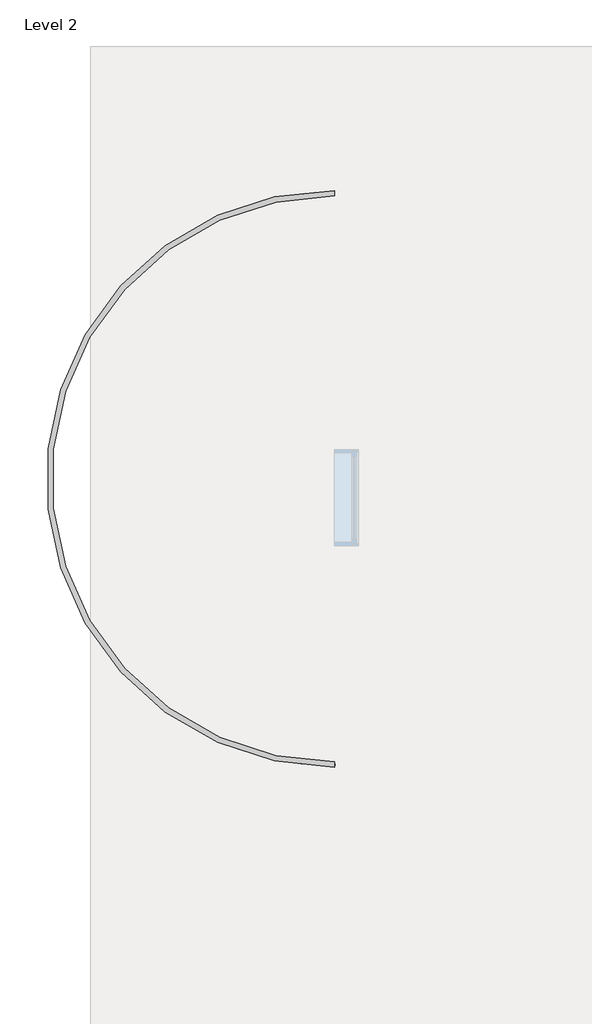
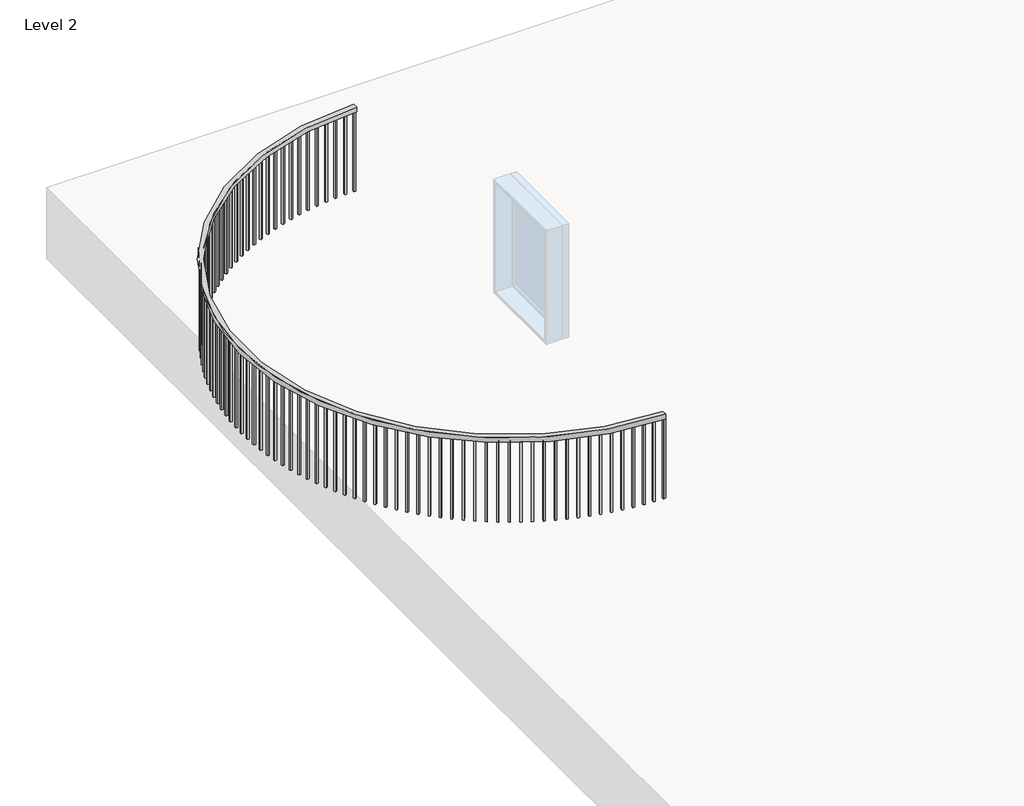
# One storey, part 2 of 2: 1 railing.
"""IFC4 building model written with IfcOpenShell, lengths in millimetres."""

from ifc_helpers import new_model, si_unit, point, frame, frame_2d, origin, place, context, project, spatial, polyline, circle_curve, trimmed, segment, composite_curve, outline, extrude, element, save

model = new_model("IFC4")

# Units and contexts
model_context = context("Model", 3, world=origin())
ifc_project = project(units=[si_unit("LENGTHUNIT", "METRE", prefix="MILLI")], contexts=[model_context])

# Site, building, storey
site = spatial("IfcSite", under=ifc_project)
building = spatial("IfcBuilding", under=site)
storey = spatial("IfcBuildingStorey", under=building, Name="Level 2", Elevation=3048.0)

# Railing
placement = place(None, origin())
element("IfcRailing", 1, ObjectType="Handrail - Rectangular", at=placement, inside=storey, context=model_context, shape_type="SweptSolid", body=[
    extrude(outline(composite_curve([segment(trimmed(circle_curve(frame_2d((-15728.6368919, 10326.9945075)), 2743.2), [point((-15728.6368919, 7583.7945075))], [point((-15728.6368919, 13070.1945075))], False, "CARTESIAN"), True, "CONTINUOUS"), segment(polyline([(-15728.6368919, 13070.1945075), (-15728.6368919, 13019.3945075)]), True, "CONTINUOUS"), segment(trimmed(circle_curve(frame_2d((-15728.6368919, 10326.9945075)), 2692.4), [point((-15728.6368919, 13019.3945075))], [point((-15728.6368919, 7634.5945075))], True, "CARTESIAN"), True, "CONTINUOUS"), segment(polyline([(-15728.6368919, 7634.5945075), (-15728.6368919, 7583.7945075)]), True, "CONTINUOUS")], self_intersect=False)), frame((0.0, 0.0, 3911.6), z_axis=(0.0, 0.0, 1.0), x_axis=(1.0, 0.0, 0.0)), (0.0, 0.0, 1.0), 50.8),
    extrude(outline(polyline([(-15741.9957848, 7599.6855919), (-15741.9690055, 7618.735573), (-15722.9190243, 7618.7087937), (-15722.9458036, 7599.6588126), (-15741.9957848, 7599.6855919)])), frame((0.0, 0.0, 3048.0), z_axis=(0.0, 0.0, 1.0), x_axis=(1.0, 0.0, 0.0)), (0.0, 0.0, 1.0), 863.6),
    extrude(outline(polyline([(-15843.9181793, 7602.0903613), (-15843.1794358, 7621.1260319), (-15824.1437651, 7620.3872884), (-15824.8825087, 7601.3516177), (-15843.9181793, 7602.0903613)])), frame((0.0, 0.0, 3048.0), z_axis=(0.0, 0.0, 1.0), x_axis=(1.0, 0.0, 0.0)), (0.0, 0.0, 1.0), 863.6),
    extrude(outline(polyline([(-15945.6794868, 7608.3027461), (-15944.2298113, 7627.297507), (-15925.2350504, 7625.8478315), (-15926.6847259, 7606.8530706), (-15945.6794868, 7608.3027461)])), frame((0.0, 0.0, 3048.0), z_axis=(0.0, 0.0, 1.0), x_axis=(1.0, 0.0, 0.0)), (0.0, 0.0, 1.0), 863.6),
    extrude(outline(polyline([(-16047.1375121, 7618.3140656), (-16044.9789303, 7637.2413746), (-16026.0516213, 7635.0827927), (-16028.2102032, 7616.1554838), (-16047.1375121, 7618.3140656)])), frame((0.0, 0.0, 3048.0), z_axis=(0.0, 0.0, 1.0), x_axis=(1.0, 0.0, 0.0)), (0.0, 0.0, 1.0), 863.6),
    extrude(outline(polyline([(-16148.150484, 7632.1103305), (-16145.2860122, 7650.9437397), (-16126.452603, 7648.0792678), (-16129.3170749, 7629.2458587), (-16148.150484, 7632.1103305)])), frame((0.0, 0.0, 3048.0), z_axis=(0.0, 0.0, 1.0), x_axis=(1.0, 0.0, 0.0)), (0.0, 0.0, 1.0), 863.6),
    extrude(outline(polyline([(-16248.5772532, 7649.6722628), (-16245.0108939, 7668.3854555), (-16226.2977012, 7664.8190963), (-16229.8640605, 7646.1059035), (-16248.5772532, 7649.6722628)])), frame((0.0, 0.0, 3048.0), z_axis=(0.0, 0.0, 1.0), x_axis=(1.0, 0.0, 0.0)), (0.0, 0.0, 1.0), 863.6),
    extrude(outline(polyline([(-16348.2774892, 7670.9753224), (-16344.014226, 7689.54215), (-16325.4473984, 7685.2788868), (-16329.7106616, 7666.7120592), (-16348.2774892, 7670.9753224)])), frame((0.0, 0.0, 3048.0), z_axis=(0.0, 0.0, 1.0), x_axis=(1.0, 0.0, 0.0)), (0.0, 0.0, 1.0), 863.6),
    extrude(outline(polyline([(-16447.1118772, 7695.9897418), (-16442.1576672, 7714.3842602), (-16423.7631489, 7709.4300502), (-16428.7173589, 7691.0355319), (-16447.1118772, 7695.9897418)])), frame((0.0, 0.0, 3048.0), z_axis=(0.0, 0.0, 1.0), x_axis=(1.0, 0.0, 0.0)), (0.0, 0.0, 1.0), 863.6),
    extrude(outline(polyline([(-16544.9423119, 7724.6805674), (-16539.3040779, 7742.8770731), (-16521.1075722, 7737.2388391), (-16526.7458062, 7719.0423334), (-16544.9423119, 7724.6805674)])), frame((0.0, 0.0, 3048.0), z_axis=(0.0, 0.0, 1.0), x_axis=(1.0, 0.0, 0.0)), (0.0, 0.0, 1.0), 863.6),
    extrude(outline(polyline([(-16641.632091, 7757.0077083), (-16635.3177115, 7774.9807746), (-16617.3446452, 7768.6663951), (-16623.6590247, 7750.6933288), (-16641.632091, 7757.0077083)])), frame((0.0, 0.0, 3048.0), z_axis=(0.0, 0.0, 1.0), x_axis=(1.0, 0.0, 0.0)), (0.0, 0.0, 1.0), 863.6),
    extrude(outline(polyline([(-16737.0461061, 7792.9259926), (-16730.0644044, 7810.6505051), (-16712.3398919, 7803.6688034), (-16719.3215936, 7785.9442909), (-16737.0461061, 7792.9259926)])), frame((0.0, 0.0, 3048.0), z_axis=(0.0, 0.0, 1.0), x_axis=(1.0, 0.0, 0.0)), (0.0, 0.0, 1.0), 863.6),
    extrude(outline(polyline([(-16831.0510314, 7832.3852302), (-16823.4117634, 7849.8364217), (-16805.9605719, 7842.1971536), (-16813.59984, 7824.7459621), (-16831.0510314, 7832.3852302)])), frame((0.0, 0.0, 3048.0), z_axis=(0.0, 0.0, 1.0), x_axis=(1.0, 0.0, 0.0)), (0.0, 0.0, 1.0), 863.6),
    extrude(outline(polyline([(-16923.5155103, 7875.3302832), (-16915.2293505, 7892.4837684), (-16898.0758652, 7884.1976086), (-16906.362025, 7867.0441234), (-16923.5155103, 7875.3302832)])), frame((0.0, 0.0, 3048.0), z_axis=(0.0, 0.0, 1.0), x_axis=(1.0, 0.0, 0.0)), (0.0, 0.0, 1.0), 863.6),
    extrude(outline(polyline([(-17014.3103383, 7921.7011427), (-17005.3888654, 7938.5329525), (-16988.5570556, 7929.6114796), (-16997.4785285, 7912.7796698), (-17014.3103383, 7921.7011427)])), frame((0.0, 0.0, 3048.0), z_axis=(0.0, 0.0, 1.0), x_axis=(1.0, 0.0, 0.0)), (0.0, 0.0, 1.0), 863.6),
    extrude(outline(polyline([(-17103.3086445, 7971.4330131), (-17093.7643247, 7987.9196276), (-17077.2777101, 7978.3753079), (-17086.8220299, 7961.8886933), (-17103.3086445, 7971.4330131)])), frame((0.0, 0.0, 3048.0), z_axis=(0.0, 0.0, 1.0), x_axis=(1.0, 0.0, 0.0)), (0.0, 0.0, 1.0), 863.6),
    extrude(outline(polyline([(-17190.3860679, 8024.4564019), (-17180.2322379, 8040.5747838), (-17164.1138559, 8030.4209539), (-17174.2676859, 8014.3025719), (-17190.3860679, 8024.4564019)])), frame((0.0, 0.0, 3048.0), z_axis=(0.0, 0.0, 1.0), x_axis=(1.0, 0.0, 0.0)), (0.0, 0.0, 1.0), 863.6),
    extrude(outline(polyline([(-17275.4209318, 8080.6972174), (-17264.67178, 8096.424844), (-17248.9441535, 8085.6756922), (-17259.6933053, 8069.9480657), (-17275.4209318, 8080.6972174)])), frame((0.0, 0.0, 3048.0), z_axis=(0.0, 0.0, 1.0), x_axis=(1.0, 0.0, 0.0)), (0.0, 0.0, 1.0), 863.6),
    extrude(outline(polyline([(-17358.2944137, 8140.0768723), (-17346.9649603, 8155.3917666), (-17331.6500661, 8144.0623132), (-17342.9795194, 8128.747419), (-17358.2944137, 8140.0768723)])), frame((0.0, 0.0, 3048.0), z_axis=(0.0, 0.0, 1.0), x_axis=(1.0, 0.0, 0.0)), (0.0, 0.0, 1.0), 863.6),
    extrude(outline(polyline([(-17438.8907113, 8202.512393), (-17426.9967874, 8217.3931549), (-17412.1160255, 8205.499231), (-17424.0099494, 8190.6184691), (-17438.8907113, 8202.512393)])), frame((0.0, 0.0, 3048.0), z_axis=(0.0, 0.0, 1.0), x_axis=(1.0, 0.0, 0.0)), (0.0, 0.0, 1.0), 863.6),
    extrude(outline(polyline([(-17517.0972041, 8267.9165359), (-17504.6554295, 8282.3423719), (-17490.2295935, 8269.9005973), (-17502.671368, 8255.4747613), (-17517.0972041, 8267.9165359)])), frame((0.0, 0.0, 3048.0), z_axis=(0.0, 0.0, 1.0), x_axis=(1.0, 0.0, 0.0)), (0.0, 0.0, 1.0), 863.6),
    extrude(outline(polyline([(-17592.8046111, 8336.1979092), (-17579.8323713, 8350.1486616), (-17565.8816189, 8337.1764217), (-17578.8538587, 8323.2256693), (-17592.8046111, 8336.1979092)])), frame((0.0, 0.0, 3048.0), z_axis=(0.0, 0.0, 1.0), x_axis=(1.0, 0.0, 0.0)), (0.0, 0.0, 1.0), 863.6),
    extrude(outline(polyline([(-17665.9071435, 8407.2611006), (-17652.422565, 8420.7172754), (-17638.9663901, 8407.2326969), (-17652.4509687, 8393.7765221), (-17665.9071435, 8407.2611006)])), frame((0.0, 0.0, 3048.0), z_axis=(0.0, 0.0, 1.0), x_axis=(1.0, 0.0, 0.0)), (0.0, 0.0, 1.0), 863.6),
    extrude(outline(polyline([(-17736.3026522, 8481.0068109), (-17722.3245775, 8493.9496053), (-17709.3817831, 8479.9715306), (-17723.3598578, 8467.0287361), (-17736.3026522, 8481.0068109)])), frame((0.0, 0.0, 3048.0), z_axis=(0.0, 0.0, 1.0), x_axis=(1.0, 0.0, 0.0)), (0.0, 0.0, 1.0), 863.6),
    extrude(outline(polyline([(-17803.8927708, 8557.3319921), (-17789.4407321, 8569.7433206), (-17777.0294035, 8555.2912819), (-17791.4814423, 8542.8799533), (-17803.8927708, 8557.3319921)])), frame((0.0, 0.0, 3048.0), z_axis=(0.0, 0.0, 1.0), x_axis=(1.0, 0.0, 0.0)), (0.0, 0.0, 1.0), 863.6),
    extrude(outline(polyline([(-17868.583053, 8636.1299922), (-17853.6772446, 8647.992512), (-17841.8147248, 8633.0867036), (-17856.7205331, 8621.2241838), (-17868.583053, 8636.1299922)])), frame((0.0, 0.0, 3048.0), z_axis=(0.0, 0.0, 1.0), x_axis=(1.0, 0.0, 0.0)), (0.0, 0.0, 1.0), 863.6),
    extrude(outline(polyline([(-17930.2831044, 8717.2907036), (-17914.9443548, 8728.5878387), (-17903.6472197, 8713.2490891), (-17918.9859693, 8701.951954), (-17930.2831044, 8717.2907036)])), frame((0.0, 0.0, 3048.0), z_axis=(0.0, 0.0, 1.0), x_axis=(1.0, 0.0, 0.0)), (0.0, 0.0, 1.0), 863.6),
    extrude(outline(polyline([(-17988.9067092, 8800.7007172), (-17973.1564519, 8811.4166817), (-17962.4404874, 8795.6664245), (-17978.1907447, 8784.9504599), (-17988.9067092, 8800.7007172)])), frame((0.0, 0.0, 3048.0), z_axis=(0.0, 0.0, 1.0), x_axis=(1.0, 0.0, 0.0)), (0.0, 0.0, 1.0), 863.6),
    extrude(outline(polyline([(-18044.3719504, 8886.2434811), (-18028.2321938, 8896.3633011), (-18018.1123738, 8880.2235446), (-18034.2521303, 8870.1037245), (-18044.3719504, 8886.2434811)])), frame((0.0, 0.0, 3048.0), z_axis=(0.0, 0.0, 1.0), x_axis=(1.0, 0.0, 0.0)), (0.0, 0.0, 1.0), 863.6),
    extrude(outline(polyline([(-18096.6013241, 8973.7994628), (-18080.094621, 8983.3089976), (-18070.5850862, 8966.8022945), (-18087.0917894, 8957.2927597), (-18096.6013241, 8973.7994628)])), frame((0.0, 0.0, 3048.0), z_axis=(0.0, 0.0, 1.0), x_axis=(1.0, 0.0, 0.0)), (0.0, 0.0, 1.0), 863.6),
    extrude(outline(polyline([(-18145.5218483, 9063.2463171), (-18128.6712641, 9072.1322785), (-18119.7853026, 9055.2816943), (-18136.6358868, 9046.3957328), (-18145.5218483, 9063.2463171)])), frame((0.0, 0.0, 3048.0), z_axis=(0.0, 0.0, 1.0), x_axis=(1.0, 0.0, 0.0)), (0.0, 0.0, 1.0), 863.6),
    extrude(outline(polyline([(-18191.0651643, 9154.4590562), (-18173.894245, 9162.7090277), (-18165.6442735, 9145.5381083), (-18182.8151929, 9137.2881369), (-18191.0651643, 9154.4590562)])), frame((0.0, 0.0, 3048.0), z_axis=(0.0, 0.0, 1.0), x_axis=(1.0, 0.0, 0.0)), (0.0, 0.0, 1.0), 863.6),
    extrude(outline(polyline([(-18233.1676328, 9247.3102252), (-18215.7003719, 9254.9126786), (-18208.0979185, 9237.4454177), (-18225.5651793, 9229.8429643), (-18233.1676328, 9247.3102252)])), frame((0.0, 0.0, 3048.0), z_axis=(0.0, 0.0, 1.0), x_axis=(1.0, 0.0, 0.0)), (0.0, 0.0, 1.0), 863.6),
    extrude(outline(polyline([(-18271.7704221, 9341.6700793), (-18254.0312274, 9348.6143915), (-18247.0869153, 9330.8751968), (-18264.82611, 9323.9308846), (-18271.7704221, 9341.6700793)])), frame((0.0, 0.0, 3048.0), z_axis=(0.0, 0.0, 1.0), x_axis=(1.0, 0.0, 0.0)), (0.0, 0.0, 1.0), 863.6),
    extrude(outline(polyline([(-18306.8195913, 9437.4067659), (-18288.8332504, 9443.6832333), (-18282.5567831, 9425.6968925), (-18300.5431239, 9419.4204251), (-18306.8195913, 9437.4067659)])), frame((0.0, 0.0, 3048.0), z_axis=(0.0, 0.0, 1.0), x_axis=(1.0, 0.0, 0.0)), (0.0, 0.0, 1.0), 863.6),
    extrude(outline(polyline([(-18338.2661646, 9534.3865084), (-18320.0578106, 9539.9863606), (-18314.4579584, 9521.7780066), (-18332.6663124, 9516.1781544), (-18338.2661646, 9534.3865084)])), frame((0.0, 0.0, 3048.0), z_axis=(0.0, 0.0, 1.0), x_axis=(1.0, 0.0, 0.0)), (0.0, 0.0, 1.0), 863.6),
    extrude(outline(polyline([(-18366.0662006, 9632.4737931), (-18347.6612768, 9637.3892053), (-18342.7458646, 9618.9842814), (-18361.1507885, 9614.0688692), (-18366.0662006, 9632.4737931)])), frame((0.0, 0.0, 3048.0), z_axis=(0.0, 0.0, 1.0), x_axis=(1.0, 0.0, 0.0)), (0.0, 0.0, 1.0), 863.6),
    extrude(outline(polyline([(-18390.1808532, 9731.5315588), (-18371.6050774, 9735.7556625), (-18367.3809737, 9717.1798866), (-18385.9567496, 9712.955783), (-18390.1808532, 9731.5315588)])), frame((0.0, 0.0, 3048.0), z_axis=(0.0, 0.0, 1.0), x_axis=(1.0, 0.0, 0.0)), (0.0, 0.0, 1.0), 863.6),
    extrude(outline(polyline([(-18410.576426, 9831.4213883), (-18391.8557549, 9834.9482809), (-18388.3288623, 9816.2276097), (-18407.0495335, 9812.7007171), (-18410.576426, 9831.4213883)])), frame((0.0, 0.0, 3048.0), z_axis=(0.0, 0.0, 1.0), x_axis=(1.0, 0.0, 0.0)), (0.0, 0.0, 1.0), 863.6),
    extrude(outline(polyline([(-18427.2244196, 9932.0037015), (-18408.3850122, 9934.8284548), (-18405.560259, 9915.9890475), (-18424.3996663, 9913.1642942), (-18427.2244196, 9932.0037015)])), frame((0.0, 0.0, 3048.0), z_axis=(0.0, 0.0, 1.0), x_axis=(1.0, 0.0, 0.0)), (0.0, 0.0, 1.0), 863.6),
    extrude(outline(polyline([(-18440.1015709, 10033.1379509), (-18421.1697524, 10035.2566177), (-18419.0510856, 10016.3247992), (-18437.9829041, 10014.2061324), (-18440.1015709, 10033.1379509)])), frame((0.0, 0.0, 3048.0), z_axis=(0.0, 0.0, 1.0), x_axis=(1.0, 0.0, 0.0)), (0.0, 0.0, 1.0), 863.6),
    extrude(outline(polyline([(-18449.1898863, 10134.6828176), (-18430.1921108, 10136.0924374), (-18428.782491, 10117.094662), (-18447.7802664, 10115.6850421), (-18449.1898863, 10134.6828176)])), frame((0.0, 0.0, 3048.0), z_axis=(0.0, 0.0, 1.0), x_axis=(1.0, 0.0, 0.0)), (0.0, 0.0, 1.0), 863.6),
    extrude(outline(polyline([(-18454.4766663, 10236.4964089), (-18435.4394802, 10237.1950121), (-18434.740877, 10218.157826), (-18453.7780631, 10217.4592228), (-18454.4766663, 10236.4964089)])), frame((0.0, 0.0, 3048.0), z_axis=(0.0, 0.0, 1.0), x_axis=(1.0, 0.0, 0.0)), (0.0, 0.0, 1.0), 863.6),
    extrude(outline(polyline([(-18455.9545234, 10338.4364568), (-18436.9045281, 10338.4230671), (-18436.9179178, 10319.3730718), (-18455.967913, 10319.3864615), (-18455.9545234, 10338.4364568)])), frame((0.0, 0.0, 3048.0), z_axis=(0.0, 0.0, 1.0), x_axis=(1.0, 0.0, 0.0)), (0.0, 0.0, 1.0), 863.6),
    extrude(outline(polyline([(-18453.6213926, 10440.3605163), (-18434.5852074, 10439.6351526), (-18435.3105712, 10420.5989673), (-18454.3467564, 10421.3243311), (-18453.6213926, 10440.3605163)])), frame((0.0, 0.0, 3048.0), z_axis=(0.0, 0.0, 1.0), x_axis=(1.0, 0.0, 0.0)), (0.0, 0.0, 1.0), 863.6),
    extrude(outline(polyline([(-18447.4805342, 10542.1261652), (-18428.4847591, 10540.6898408), (-18429.9210834, 10521.6940657), (-18448.9168585, 10523.13039), (-18447.4805342, 10542.1261652)])), frame((0.0, 0.0, 3048.0), z_axis=(0.0, 0.0, 1.0), x_axis=(1.0, 0.0, 0.0)), (0.0, 0.0, 1.0), 863.6),
    extrude(outline(polyline([(-18437.5405288, 10643.5912021), (-18418.6117074, 10641.4459242), (-18420.7569852, 10622.5171027), (-18439.6858067, 10624.6623806), (-18437.5405288, 10643.5912021)])), frame((0.0, 0.0, 3048.0), z_axis=(0.0, 0.0, 1.0), x_axis=(1.0, 0.0, 0.0)), (0.0, 0.0, 1.0), 863.6),
    extrude(outline(polyline([(-18423.8152662, 10744.613846), (-18404.9798483, 10741.7626123), (-18407.8310821, 10722.9271944), (-18426.6664999, 10725.7784281), (-18423.8152662, 10744.613846)])), frame((0.0, 0.0, 3048.0), z_axis=(0.0, 0.0, 1.0), x_axis=(1.0, 0.0, 0.0)), (0.0, 0.0, 1.0), 863.6),
    extrude(outline(polyline([(-18406.3239251, 10845.0529341), (-18387.6082304, 10841.4997286), (-18391.1614358, 10822.7840338), (-18409.8771306, 10826.3372393), (-18406.3239251, 10845.0529341)])), frame((0.0, 0.0, 3048.0), z_axis=(0.0, 0.0, 1.0), x_axis=(1.0, 0.0, 0.0)), (0.0, 0.0, 1.0), 863.6),
    extrude(outline(polyline([(-18385.0909469, 10944.7681188), (-18366.5211274, 10940.5179066), (-18370.7713395, 10921.9480871), (-18389.341159, 10926.1982992), (-18385.0909469, 10944.7681188)])), frame((0.0, 0.0, 3048.0), z_axis=(0.0, 0.0, 1.0), x_axis=(1.0, 0.0, 0.0)), (0.0, 0.0, 1.0), 863.6),
    extrude(outline(polyline([(-18360.1460013, 11043.6200641), (-18341.7480054, 11038.6787843), (-18346.6892852, 11020.2807884), (-18365.0872811, 11025.2220682), (-18360.1460013, 11043.6200641)])), frame((0.0, 0.0, 3048.0), z_axis=(0.0, 0.0, 1.0), x_axis=(1.0, 0.0, 0.0)), (0.0, 0.0, 1.0), 863.6),
    extrude(outline(polyline([(-18331.5239448, 11141.4706405), (-18313.3234807, 11135.8451977), (-18318.9489235, 11117.6447336), (-18337.1493876, 11123.2701765), (-18331.5239448, 11141.4706405)])), frame((0.0, 0.0, 3048.0), z_axis=(0.0, 0.0, 1.0), x_axis=(1.0, 0.0, 0.0)), (0.0, 0.0, 1.0), 863.6),
    extrude(outline(polyline([(-18299.2647721, 11238.1831175), (-18281.287272, 11231.8813723), (-18287.5890173, 11213.9038722), (-18305.5665173, 11220.2056175), (-18299.2647721, 11238.1831175)])), frame((0.0, 0.0, 3048.0), z_axis=(0.0, 0.0, 1.0), x_axis=(1.0, 0.0, 0.0)), (0.0, 0.0, 1.0), 863.6),
    extrude(outline(polyline([(-18263.4135602, 11333.6223549), (-18245.6841449, 11326.6531129), (-18252.6533869, 11308.9236976), (-18270.3828021, 11315.8929396), (-18263.4135602, 11333.6223549)])), frame((0.0, 0.0, 3048.0), z_axis=(0.0, 0.0, 1.0), x_axis=(1.0, 0.0, 0.0)), (0.0, 0.0, 1.0), 863.6),
    extrude(outline(polyline([(-18224.0204055, 11427.6549917), (-18206.5638489, 11420.0279914), (-18214.1908492, 11402.5714348), (-18231.6474057, 11410.1984351), (-18224.0204055, 11427.6549917)])), frame((0.0, 0.0, 3048.0), z_axis=(0.0, 0.0, 1.0), x_axis=(1.0, 0.0, 0.0)), (0.0, 0.0, 1.0), 863.6),
    extrude(outline(polyline([(-18181.1403535, 11520.1496324), (-18163.9810484, 11511.8755313), (-18172.2551495, 11494.7162262), (-18189.4144546, 11502.9903273), (-18181.1403535, 11520.1496324)])), frame((0.0, 0.0, 3048.0), z_axis=(0.0, 0.0, 1.0), x_axis=(1.0, 0.0, 0.0)), (0.0, 0.0, 1.0), 863.6),
    extrude(outline(polyline([(-18134.8333222, 11610.9770307), (-18117.995246, 11602.0673905), (-18126.9048862, 11585.2293142), (-18143.7429624, 11594.1389544), (-18134.8333222, 11610.9770307)])), frame((0.0, 0.0, 3048.0), z_axis=(0.0, 0.0, 1.0), x_axis=(1.0, 0.0, 0.0)), (0.0, 0.0, 1.0), 863.6),
    extrude(outline(polyline([(-18085.1640183, 11700.0102698), (-18068.6706994, 11690.4775403), (-18078.2034289, 11673.9842214), (-18094.6967478, 11683.5169509), (-18085.1640183, 11700.0102698)])), frame((0.0, 0.0, 3048.0), z_axis=(0.0, 0.0, 1.0), x_axis=(1.0, 0.0, 0.0)), (0.0, 0.0, 1.0), 863.6),
    extrude(outline(polyline([(-18032.2018467, 11787.1249402), (-18016.0763318, 11776.9824419), (-18026.2188302, 11760.8569271), (-18042.344345, 11770.9994254), (-18032.2018467, 11787.1249402)])), frame((0.0, 0.0, 3048.0), z_axis=(0.0, 0.0, 1.0), x_axis=(1.0, 0.0, 0.0)), (0.0, 0.0, 1.0), 863.6),
    extrude(outline(polyline([(-17976.0208133, 11872.199313), (-17960.2856354, 11861.4612184), (-17971.0237301, 11845.7260405), (-17986.758908, 11856.4641351), (-17976.0208133, 11872.199313)])), frame((0.0, 0.0, 3048.0), z_axis=(0.0, 0.0, 1.0), x_axis=(1.0, 0.0, 0.0)), (0.0, 0.0, 1.0), 863.6),
    extrude(outline(polyline([(-17916.6994223, 11955.1145106), (-17901.3765687, 11943.7958244), (-17912.6952549, 11928.4729708), (-17928.0181085, 11939.791657), (-17916.6994223, 11955.1145106)])), frame((0.0, 0.0, 3048.0), z_axis=(0.0, 0.0, 1.0), x_axis=(1.0, 0.0, 0.0)), (0.0, 0.0, 1.0), 863.6),
    extrude(outline(polyline([(-17854.3205656, 12035.7546722), (-17839.4314475, 12023.8712105), (-17851.3149093, 12008.9820924), (-17866.2040274, 12020.8655541), (-17854.3205656, 12035.7546722)])), frame((0.0, 0.0, 3048.0), z_axis=(0.0, 0.0, 1.0), x_axis=(1.0, 0.0, 0.0)), (0.0, 0.0, 1.0), 863.6),
    extrude(outline(polyline([(-17788.9714078, 12114.0071162), (-17774.5368304, 12101.5754842), (-17786.9684624, 12087.1409068), (-17801.4030399, 12099.5725388), (-17788.9714078, 12114.0071162)])), frame((0.0, 0.0, 3048.0), z_axis=(0.0, 0.0, 1.0), x_axis=(1.0, 0.0, 0.0)), (0.0, 0.0, 1.0), 863.6),
    extrude(outline(polyline([(-17720.7432638, 12189.7624974), (-17706.783397, 12176.8000663), (-17719.7458282, 12162.8401996), (-17733.7056949, 12175.8026307), (-17720.7432638, 12189.7624974)])), frame((0.0, 0.0, 3048.0), z_axis=(0.0, 0.0, 1.0), x_axis=(1.0, 0.0, 0.0)), (0.0, 0.0, 1.0), 863.6),
    extrude(outline(polyline([(-17649.7314714, 12262.9149599), (-17636.265822, 12249.4398426), (-17649.7409393, 12235.9741932), (-17663.2065887, 12249.4493105), (-17649.7314714, 12262.9149599)])), frame((0.0, 0.0, 3048.0), z_axis=(0.0, 0.0, 1.0), x_axis=(1.0, 0.0, 0.0)), (0.0, 0.0, 1.0), 863.6),
    extrude(outline(polyline([(-17576.0352582, 12333.3622847), (-17563.0826422, 12319.3933106), (-17577.0516164, 12306.4406946), (-17590.0042323, 12320.4096688), (-17576.0352582, 12333.3622847)])), frame((0.0, 0.0, 3048.0), z_axis=(0.0, 0.0, 1.0), x_axis=(1.0, 0.0, 0.0)), (0.0, 0.0, 1.0), 863.6),
    extrude(outline(polyline([(-17499.7576028, 12401.0060332), (-17487.3361194, 12386.5627216), (-17501.779431, 12374.1412382), (-17514.2009144, 12388.5845499), (-17499.7576028, 12401.0060332)])), frame((0.0, 0.0, 3048.0), z_axis=(0.0, 0.0, 1.0), x_axis=(1.0, 0.0, 0.0)), (0.0, 0.0, 1.0), 863.6),
    extrude(outline(polyline([(-17421.0050909, 12465.751684), (-17409.1320972, 12450.8542171), (-17424.0295641, 12438.9812234), (-17435.9025578, 12453.8786903), (-17421.0050909, 12465.751684)])), frame((0.0, 0.0, 3048.0), z_axis=(0.0, 0.0, 1.0), x_axis=(1.0, 0.0, 0.0)), (0.0, 0.0, 1.0), 863.6),
    extrude(outline(polyline([(-17339.8877666, 12527.5087656), (-17328.5798531, 12512.1779602), (-17343.9106585, 12500.8700467), (-17355.218572, 12516.2008521), (-17339.8877666, 12527.5087656)])), frame((0.0, 0.0, 3048.0), z_axis=(0.0, 0.0, 1.0), x_axis=(1.0, 0.0, 0.0)), (0.0, 0.0, 1.0), 863.6),
    extrude(outline(polyline([(-17256.5189783, 12586.1909822), (-17245.791946, 12570.4482607), (-17261.5346675, 12559.7212285), (-17272.2616997, 12575.46395), (-17256.5189783, 12586.1909822)])), frame((0.0, 0.0, 3048.0), z_axis=(0.0, 0.0, 1.0), x_axis=(1.0, 0.0, 0.0)), (0.0, 0.0, 1.0), 863.6),
    extrude(outline(polyline([(-17171.0152203, 12641.716335), (-17160.8840587, 12625.5836953), (-17177.0166983, 12615.4525337), (-17187.14786, 12631.5851733), (-17171.0152203, 12641.716335)])), frame((0.0, 0.0, 3048.0), z_axis=(0.0, 0.0, 1.0), x_axis=(1.0, 0.0, 0.0)), (0.0, 0.0, 1.0), 863.6),
    extrude(outline(polyline([(-17083.4959706, 12694.0072362), (-17073.9748361, 12677.5072211), (-17090.4748512, 12667.9860867), (-17099.9959857, 12684.4861018), (-17083.4959706, 12694.0072362)])), frame((0.0, 0.0, 3048.0), z_axis=(0.0, 0.0, 1.0), x_axis=(1.0, 0.0, 0.0)), (0.0, 0.0, 1.0), 863.6),
    extrude(outline(polyline([(-16994.0835232, 12742.9906177), (-16985.1857201, 12726.1462833), (-17002.0300546, 12717.2484803), (-17010.9278576, 12734.0928147), (-16994.0835232, 12742.9906177)])), frame((0.0, 0.0, 3048.0), z_axis=(0.0, 0.0, 1.0), x_axis=(1.0, 0.0, 0.0)), (0.0, 0.0, 1.0), 863.6),
    extrude(outline(polyline([(-16902.9028175, 12788.5980331), (-16894.6407792, 12771.4329166), (-16911.8058957, 12763.1708783), (-16920.067934, 12780.3359948), (-16902.9028175, 12788.5980331)])), frame((0.0, 0.0, 3048.0), z_axis=(0.0, 0.0, 1.0), x_axis=(1.0, 0.0, 0.0)), (0.0, 0.0, 1.0), 863.6),
    extrude(outline(polyline([(-16810.081264, 12830.7657533), (-16802.4665353, 12813.3038403), (-16819.9284483, 12805.6891115), (-16827.543177, 12823.1510246), (-16810.081264, 12830.7657533)])), frame((0.0, 0.0, 3048.0), z_axis=(0.0, 0.0, 1.0), x_axis=(1.0, 0.0, 0.0)), (0.0, 0.0, 1.0), 863.6),
    extrude(outline(polyline([(-16715.7485659, 12869.4348557), (-16708.7917871, 12851.7005464), (-16726.5260965, 12844.7437676), (-16733.4828752, 12862.4780769), (-16715.7485659, 12869.4348557)])), frame((0.0, 0.0, 3048.0), z_axis=(0.0, 0.0, 1.0), x_axis=(1.0, 0.0, 0.0)), (0.0, 0.0, 1.0), 863.6),
    extrude(outline(polyline([(-16620.0365379, 12904.5513065), (-16613.74743, 12886.5693817), (-16631.7293549, 12880.2802738), (-16638.0184627, 12898.2621987), (-16620.0365379, 12904.5513065)])), frame((0.0, 0.0, 3048.0), z_axis=(0.0, 0.0, 1.0), x_axis=(1.0, 0.0, 0.0)), (0.0, 0.0, 1.0), 863.6),
    extrude(outline(polyline([(-16523.0789222, 12936.0660362), (-16517.4662733, 12917.8616226), (-16535.6706868, 12912.2489737), (-16541.2833357, 12930.4533872), (-16523.0789222, 12936.0660362)])), frame((0.0, 0.0, 3048.0), z_axis=(0.0, 0.0, 1.0), x_axis=(1.0, 0.0, 0.0)), (0.0, 0.0, 1.0), 863.6),
    extrude(outline(polyline([(-16425.0112015, 12963.9350078), (-16420.0828543, 12945.5335433), (-16438.4843187, 12940.6051961), (-16443.4126659, 12959.0066606), (-16425.0112015, 12963.9350078)])), frame((0.0, 0.0, 3048.0), z_axis=(0.0, 0.0, 1.0), x_axis=(1.0, 0.0, 0.0)), (0.0, 0.0, 1.0), 863.6),
    extrude(outline(polyline([(-16325.9704097, 12988.119279), (-16321.7332507, 12969.5464768), (-16340.306053, 12965.3093178), (-16344.5432119, 12983.8821201), (-16325.9704097, 12988.119279)])), frame((0.0, 0.0, 3048.0), z_axis=(0.0, 0.0, 1.0), x_axis=(1.0, 0.0, 0.0)), (0.0, 0.0, 1.0), 863.6),
    extrude(outline(polyline([(-16226.0949403, 13008.5850563), (-16222.5548904, 12989.8668687), (-16241.273078, 12986.3268188), (-16244.8131279, 13005.0450064), (-16226.0949403, 13008.5850563)])), frame((0.0, 0.0, 3048.0), z_axis=(0.0, 0.0, 1.0), x_axis=(1.0, 0.0, 0.0)), (0.0, 0.0, 1.0), 863.6),
    extrude(outline(polyline([(-16125.5243533, 13025.3037418), (-16122.686359, 13006.4663246), (-16141.5237763, 13003.6283304), (-16144.3617705, 13022.4657476), (-16125.5243533, 13025.3037418)])), frame((0.0, 0.0, 3048.0), z_axis=(0.0, 0.0, 1.0), x_axis=(1.0, 0.0, 0.0)), (0.0, 0.0, 1.0), 863.6),
    extrude(outline(polyline([(-16024.3991798, 13038.2519741), (-16022.2672069, 13019.3216494), (-16041.1975316, 13017.1896766), (-16043.3295045, 13036.1200012), (-16024.3991798, 13038.2519741)])), frame((0.0, 0.0, 3048.0), z_axis=(0.0, 0.0, 1.0), x_axis=(1.0, 0.0, 0.0)), (0.0, 0.0, 1.0), 863.6),
    extrude(outline(polyline([(-15922.8607261, 13047.41166), (-15921.4377537, 13028.41488), (-15940.4345336, 13026.9919075), (-15941.8575061, 13045.9886875), (-15922.8607261, 13047.41166)])), frame((0.0, 0.0, 3048.0), z_axis=(0.0, 0.0, 1.0), x_axis=(1.0, 0.0, 0.0)), (0.0, 0.0, 1.0), 863.6),
    extrude(outline(polyline([(-15821.0508759, 13052.7700002), (-15820.3388922, 13033.7333099), (-15839.3755825, 13033.0213262), (-15840.0875662, 13052.0580165), (-15821.0508759, 13052.7700002)])), frame((0.0, 0.0, 3048.0), z_axis=(0.0, 0.0, 1.0), x_axis=(1.0, 0.0, 0.0)), (0.0, 0.0, 1.0), 863.6),
    extrude(outline(polyline([(-15747.7201959, 7599.7196389), (-15747.653432, 7618.7695219), (-15728.603549, 7618.702758), (-15728.6703128, 7599.652875), (-15747.7201959, 7599.7196389)])), frame((0.0, 0.0, 3048.0), z_axis=(0.0, 0.0, 1.0), x_axis=(1.0, 0.0, 0.0)), (0.0, 0.0, 1.0), 863.6),
    extrude(outline(polyline([(-15728.6703128, 13054.3361399), (-15728.603549, 13035.2862569), (-15747.653432, 13035.219493), (-15747.7201959, 13054.2693761), (-15728.6703128, 13054.3361399)])), frame((0.0, 0.0, 3048.0), z_axis=(0.0, 0.0, 1.0), x_axis=(1.0, 0.0, 0.0)), (0.0, 0.0, 1.0), 863.6),
])

save(model, "model.ifc")

# Revit data of these elements
# Type "Handrail - Rectangular"
#   Assembly Code = "C2010400"
#   built-in parameter 1008612 = 0.0416667 (stored number, unit not read)
#   built-in parameter 1008611 = 0.0416667 (stored number, unit not read)
#   built-in parameter 1008609 = 0.333333 (stored number, unit not read)
#   built-in parameter 1008604 = 0.166667 (stored number, unit not read)
#   built-in parameter 1008603 = 0.166667 (stored number, unit not read)
#   Railing Height = 3' - 0"
#   built-in parameter 1008630 = 2
#   built-in parameter 1008610 = 2
#   built-in parameter 1008618 = Baluster - Square : 3/4"
# Element 1 (IfcRailing, "Handrail - Rectangular")
#   Phase Created = New Construction
